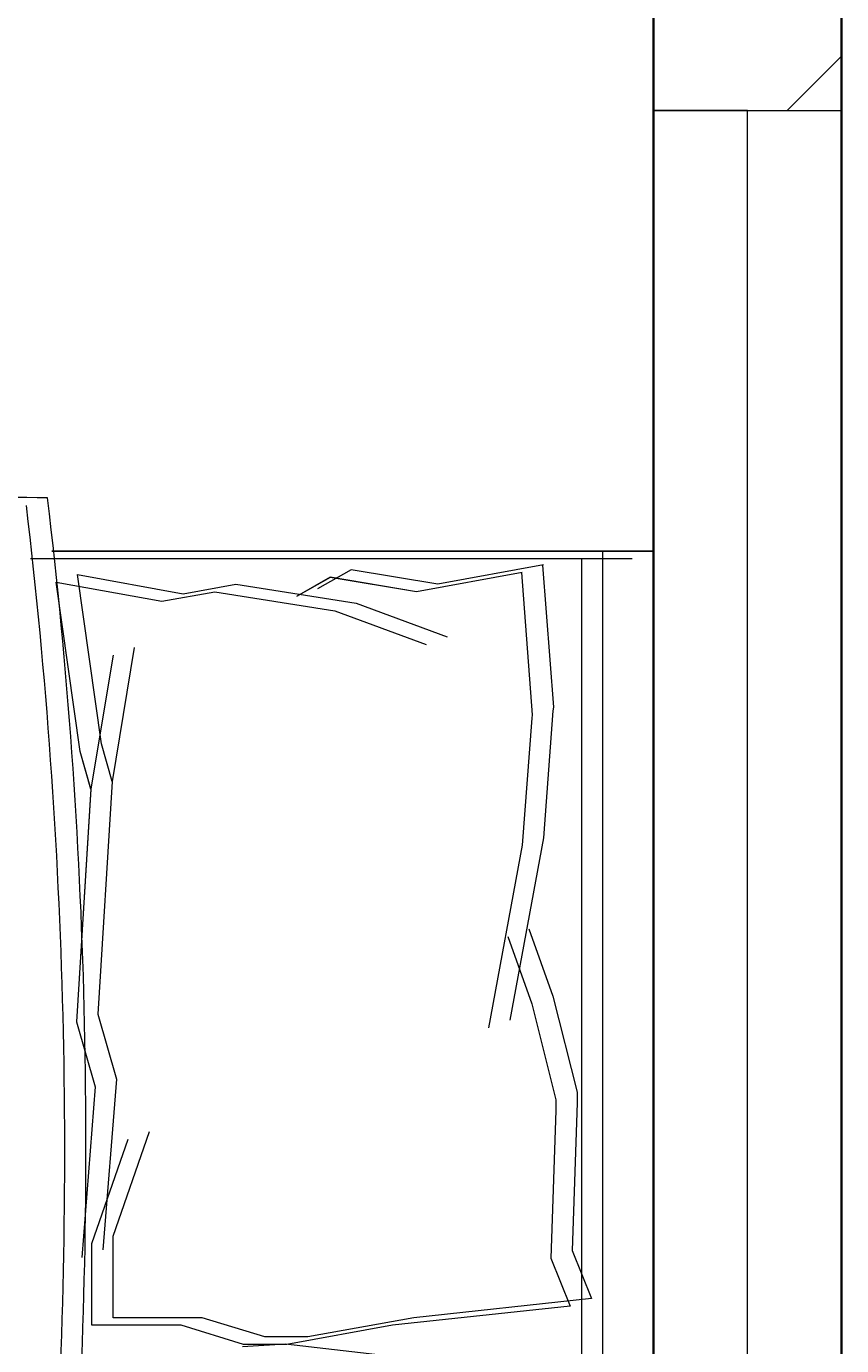
# Model space of a CAD drawing. Units: inches. Extents: x 1962 to 2771, y 1245 to 2660.
# Tile 77 of 114: x 2641 to 2661, y 2051 to 2082. Entities that reach past the tile are written whole.
import ezdxf

# ---------------------------------------------------------------- set-up
doc = ezdxf.new("R2010")
doc.units = ezdxf.units.IN
for name, color, linetype, lineweight in [('A-ANNO-DIMS', 2, 'Continuous', 18), ('A-FURN', 8, 'Continuous', 13), ('A-GLAZ', 4, 'Continuous', 18), ('A-WALL', 7, 'Continuous', 35), ('A-WALL-PATT', 252, 'Continuous', 13)]:
    doc.layers.add(name, color=color, linetype=linetype, lineweight=lineweight)
doc.styles.get("Standard").update_dxf_attribs({"font": 'arial.ttf'})
doc.dimstyles.get("Standard").update_dxf_attribs({"dimtxt": 0.18, "dimasz": 0.18, "dimexe": 0.18, "dimexo": 0.0625, "dimgap": 0.09, "dimtad": 0, "dimtih": 1, "dimtoh": 1, "dimdec": 4, "dimzin": 0, "dimdsep": 46, "dimtxsty": 'Standard', "dimcen": 0.09, "dimadec": 0, "dimazin": 0, "dimtfac": 1, "dimtdec": 4, "dimtofl": 0, "dimtmove": 0, "dimatfit": 3, "dimfxl": 1, "dimtolj": 1, "dimtzin": 0, "dimarcsym": 0})

# ---------------------------------------------------------------- blocks, each defined once
blk = doc.blocks.new('BED-PLAN')
for p, q in [((0, 2.764), (0, 40.751)), ((1.219, 2.764), (1.219, 40.752)), ((1.219, 2.763), (1.219, 40.751)), ((1.727, 2.945), (1.727, 40.933)), ((1.727, 2.945), (1.727, 40.933)), ((6.254, 22.046), (8.806, 21.745)), ((6.254, 22.046), (8.806, 21.745)), ((8.806, 21.745), (9.838, 21.81)), ((8.806, 21.745), (9.838, 21.81)), ((5.739, 21.114), (8.268, 21.574)), ((5.739, 21.114), (8.268, 21.574)), ((6.247, 21.296), (8.776, 21.755)), ((6.247, 21.296), (8.776, 21.755)), ((8.268, 21.574), (9.302, 21.574)), ((8.268, 21.574), (9.302, 21.574)), ((8.776, 21.755), (9.81, 21.755)), ((8.776, 21.755), (9.81, 21.755)), ((9.302, 21.574), (10.796, 21.114)), ((9.302, 21.574), (10.796, 21.114)), ((9.81, 21.755), (11.304, 21.296)), ((9.81, 21.755), (11.304, 21.296)), ((1.995, 20.836), (6.247, 21.296)), ((1.995, 20.836), (6.247, 21.296)), ((11.304, 21.296), (13.436, 21.296)), ((11.304, 21.296), (13.436, 21.296)), ((13.436, 21.296), (13.436, 19.342)), ((13.436, 21.296), (13.436, 19.342)), ((1.487, 20.655), (5.739, 21.114)), ((1.487, 20.654), (5.739, 21.114)), ((10.796, 21.114), (12.927, 21.114)), ((10.796, 21.114), (12.927, 21.114)), ((12.927, 21.114), (12.927, 19.161)), ((12.927, 21.114), (12.927, 19.161)), ((1.946, 19.506), (1.487, 20.655)), ((1.946, 19.505), (1.487, 20.654)), ((2.455, 19.687), (1.995, 20.836)), ((2.455, 19.687), (1.995, 20.836)), ((2.34, 16.153), (2.455, 19.687)), ((2.34, 16.153), (2.455, 19.687)), ((13.361, 15.591), (13.682, 19.67)), ((13.361, 15.591), (13.682, 19.67)), ((1.831, 15.972), (1.946, 19.506)), ((1.831, 15.972), (1.946, 19.505)), ((13.436, 19.342), (12.568, 16.843)), ((13.436, 19.342), (12.568, 16.843)), ((12.853, 15.409), (13.173, 19.489)), ((12.853, 15.409), (13.173, 19.488)), ((12.927, 19.161), (12.06, 16.661)), ((12.927, 19.161), (12.06, 16.661)), ((2.34, 15.898), (2.34, 16.153)), ((2.34, 15.897), (2.34, 16.153)), ((1.831, 15.716), (1.831, 15.972)), ((1.831, 15.716), (1.831, 15.972)), ((2.914, 13.6), (2.34, 15.898)), ((2.914, 13.599), (2.34, 15.897)), ((2.406, 13.418), (1.831, 15.716)), ((2.406, 13.418), (1.831, 15.716)), ((13.804, 14.033), (13.361, 15.591)), ((13.804, 14.032), (13.361, 15.591)), ((13.296, 13.851), (12.853, 15.409)), ((13.296, 13.851), (12.853, 15.409)), ((2.636, 9.626), (3.44, 13.993)), ((2.636, 9.626), (3.44, 13.992)), ((3.144, 9.808), (3.949, 14.174)), ((3.144, 9.807), (3.949, 14.174)), ((13.461, 8.461), (13.804, 14.033)), ((13.461, 8.46), (13.804, 14.032)), ((3.489, 11.991), (2.914, 13.6)), ((3.489, 11.991), (2.914, 13.599)), ((12.953, 8.279), (13.296, 13.851)), ((12.953, 8.279), (13.296, 13.851)), ((2.981, 11.809), (2.406, 13.418)), ((2.981, 11.809), (2.406, 13.418)), ((2.914, 6.768), (3.144, 9.808)), ((2.914, 6.768), (3.144, 9.807)), ((2.406, 6.587), (2.636, 9.626)), ((2.406, 6.587), (2.636, 9.626)), ((12.423, 5.074), (12.953, 8.279)), ((12.423, 5.074), (12.953, 8.279)), ((12.931, 5.256), (13.461, 8.461)), ((12.931, 5.255), (13.461, 8.46)), ((12.953, 8.279), (13.21, 7.378)), ((12.953, 8.279), (13.21, 7.378)), ((13.461, 8.461), (13.718, 7.56)), ((13.461, 8.46), (13.718, 7.56)), ((13.21, 7.378), (13.784, 3.327)), ((13.21, 7.378), (13.784, 3.327)), ((13.718, 7.56), (14.292, 3.509)), ((13.718, 7.56), (14.292, 3.508)), ((2.9, 6.685), (2.914, 6.768)), ((2.9, 6.684), (2.914, 6.768)), ((3.162, 3.282), (2.9, 6.685)), ((3.162, 3.282), (2.9, 6.684)), ((2.392, 6.503), (2.406, 6.587)), ((2.392, 6.503), (2.406, 6.587)), ((2.653, 3.1), (2.392, 6.503)), ((2.653, 3.1), (2.392, 6.503)), ((7.118, 4.016), (4.935, 4.821)), ((7.118, 4.016), (4.935, 4.821)), ((7.626, 4.198), (5.443, 5.002)), ((7.626, 4.198), (5.443, 5.002)), ((10.5, 3.738), (7.626, 4.198)), ((10.5, 3.738), (7.626, 4.198)), ((9.991, 3.557), (7.118, 4.016)), ((9.992, 3.557), (7.118, 4.016)), ((7.741, 3.394), (8.546, 3.853)), ((7.741, 3.393), (8.546, 3.853)), ((11.764, 3.968), (10.5, 3.738)), ((11.764, 3.968), (10.5, 3.738)), ((14.292, 3.509), (11.764, 3.968)), ((14.292, 3.508), (11.764, 3.968)), ((2.636, 3.097), (5.164, 3.557)), ((2.636, 3.097), (5.164, 3.557)), ((3.144, 3.279), (5.673, 3.738)), ((3.144, 3.279), (5.673, 3.738)), ((5.164, 3.557), (7.233, 3.212)), ((5.164, 3.557), (7.233, 3.212)), ((5.673, 3.738), (7.741, 3.394)), ((5.673, 3.738), (7.741, 3.393)), ((7.233, 3.212), (8.038, 3.672)), ((7.233, 3.212), (8.038, 3.672)), ((11.256, 3.787), (9.991, 3.557)), ((11.256, 3.786), (9.992, 3.557)), ((13.784, 3.327), (11.256, 3.787)), ((13.784, 3.327), (11.256, 3.786)), ((14.904, 2.945), (0.508, 2.945)), ((14.904, 2.945), (0.508, 2.945)), ((14.396, 2.764), (0, 2.764)), ((14.396, 2.763), (0, 2.763))]:
    blk.add_line(p, q)
for centre, radius, start, end in [((144.711, 16.979), 131.131, 176.08655, 186.78213), ((144.711, 16.979), 131.131, 176.08655, 186.78213), ((145.219, 17.161), 131.131, 176.08655, 186.78213), ((145.219, 17.161), 131.131, 176.08655, 186.78213), ((15.974, 67.695), 66.218, 268.72178, 275.60397), ((15.974, 67.695), 66.218, 268.72178, 275.60397)]:
    blk.add_arc(centre, radius, start, end)
blk = doc.blocks.new('WIN-60IN-A')
for p, q in [((2.25, 60), (2.25, 0)), ((2.25, 0), (0, 0)), ((0, 0), (4.5, 0))]:
    blk.add_line(p, q)
blk = doc.blocks.new('*D40')
at = {"layer": 'A-ANNO-DIMS', "color": 0, "lineweight": -2, "transparency": 16777216}
for p, q in [((2072.02, 2033.906), (2072.02, 2583.474)), ((2072.2, 2583.294), (2366.02, 2583.294)), ((2660.627, 2583.294), (2366.808, 2583.294)), ((2660.807, 2524.406), (2660.807, 2583.474))]:
    blk.add_line(p, q, dxfattribs=at)
at = {"layer": 'A-ANNO-DIMS', "color": 0, "transparency": 16777216}
for points in [[(2072.2, 2583.324), (2072.2, 2583.264), (2072.02, 2583.294)], [(2660.627, 2583.324), (2660.627, 2583.264), (2660.807, 2583.294)]]:
    blk.add_solid(points, dxfattribs=at)
at = {"layer": 'Defpoints', "color": 0, "transparency": 16777216}
for p in [(2660.807, 2583.294), (2660.807, 2524.344), (2072.02, 2033.844)]:
    blk.add_point(p, dxfattribs=at)
at = {"layer": 'A-ANNO-DIMS', "color": 0, "transparency": 16777216, "insert": (2366.414, 2583.294), "char_height": 0.18, "attachment_point": 5}
blk.add_mtext('\\A1;588.8', dxfattribs=at)

msp = doc.modelspace()

# ---------------------------------------------------------------- hatches: boundary and pattern name
at = {"layer": 'A-WALL-PATT'}
h = msp.add_hatch(dxfattribs=at)
h.set_pattern_fill('ANSI32', color=256)
h.paths.add_polyline_path([(2090.8074, 2467.3437), (2141.6481, 2467.3437), (2141.6481, 2469.5937), (2141.6481, 2471.8437), (2086.3074, 2471.8437), (2086.3074, 2422.5333), (2090.8074, 2422.5333)])
h.paths.add_polyline_path([(2282.7664, 2471.8437), (2204.8982, 2471.8437), (2204.8982, 2467.3437), (2234.8074, 2467.3437), (2234.8074, 2311.3437), (2228.7492, 2311.3437), (2228.7492, 2306.8437), (2234.8074, 2306.8437), (2331.9227, 2306.8437), (2331.9227, 2309.0937), (2331.9227, 2311.3437), (2239.3074, 2311.3437), (2239.3074, 2467.3437), (2282.7664, 2467.3437), (2282.7664, 2469.5937)])
h.paths.add_polyline_path([(2471.4531, 2519.8437), (2552.011, 2519.8437), (2564.3996, 2519.8437), (2564.3996, 2511.1389), (2568.8996, 2511.1389), (2568.8996, 2524.3437), (2466.9531, 2524.3437), (2466.9531, 2471.8437), (2450.0749, 2471.8437), (2446.4672, 2471.8437), (2446.4672, 2467.3437), (2450.0749, 2467.3437), (2475.9988, 2467.3437), (2475.9988, 2469.5937), (2475.9988, 2471.8437), (2471.4531, 2471.8437)])
h.paths.add_polyline_path([(2575.2231, 2469.5937), (2575.2231, 2471.8437), (2568.8996, 2471.8437), (2568.8996, 2487.1389), (2564.3996, 2487.1389), (2564.3996, 2471.8437), (2556.511, 2471.8437), (2499.2904, 2471.8437), (2499.2904, 2467.3437), (2507.8074, 2467.3437), (2507.8074, 2311.3437), (2414.863, 2311.3437), (2414.863, 2306.8437), (2512.3074, 2306.8437), (2517.0114, 2306.8437), (2517.0114, 2309.0937), (2517.0114, 2311.3437), (2512.3074, 2311.3437), (2512.3074, 2467.3437), (2575.2231, 2467.3437)])
h.paths.add_polyline_path([(2660.8074, 2471.8437), (2600.9602, 2471.8437), (2600.9602, 2467.3437), (2656.3074, 2467.3437), (2656.3074, 2432.5704), (2660.8074, 2432.5704)])
h.paths.add_polyline_path([(2660.8074, 2372.5704), (2656.3074, 2372.5704), (2656.3074, 2311.3437), (2600.276, 2311.3437), (2600.276, 2309.0937), (2600.276, 2306.8437), (2656.3074, 2306.8437), (2656.3074, 2296.2593), (2660.8074, 2296.2593)])
h.paths.add_polyline_path([(2572.3074, 2306.8437), (2577.1385, 2306.8437), (2577.1385, 2311.3437), (2551.082, 2311.3437), (2551.082, 2306.8437), (2567.8074, 2306.8437), (2567.8074, 2258.8437), (2540.0574, 2258.8437), (2540.0574, 2256.5937), (2540.0574, 2254.3437), (2567.8074, 2254.3437), (2656.3074, 2254.3437), (2656.3074, 2236.9085), (2660.8074, 2236.9085), (2660.8074, 2272.2593), (2656.3074, 2272.2593), (2656.3074, 2258.8437), (2572.3074, 2258.8437)])
h.paths.add_polyline_path([(2512.3074, 2254.3437), (2518.8716, 2254.3437), (2518.8716, 2256.5937), (2518.8716, 2258.8437), (2507.8074, 2258.8437), (2507.8074, 2177.8437), (2567.8074, 2177.8437), (2567.8074, 2172.9628), (2572.3074, 2172.9628), (2572.3074, 2177.8437), (2656.3074, 2177.8437), (2656.3074, 2166.4846), (2660.8074, 2166.4846), (2660.8074, 2200.9085), (2656.3074, 2200.9085), (2656.3074, 2182.3437), (2512.3074, 2182.3437)])
h.paths.add_polyline_path([(2656.3074, 2129.8437), (2572.3074, 2129.8437), (2572.3074, 2150.3044), (2570.0574, 2150.3044), (2567.8074, 2150.3044), (2567.8074, 2129.8437), (2507.8074, 2129.8437), (2507.8074, 2116.3027), (2510.0574, 2116.3027), (2512.3074, 2116.3027), (2512.3074, 2125.3437), (2567.8074, 2125.3437), (2572.3074, 2125.3437), (2656.3074, 2125.3437)])
h.paths.add_polyline_path([(2090.8074, 2362.5333), (2086.3074, 2362.5333), (2086.3074, 2298.6242), (2090.8074, 2298.6242), (2090.8074, 2306.8437), (2174.8074, 2306.8437), (2174.8074, 2286.4178), (2179.3074, 2286.4178), (2179.3074, 2306.8437), (2192.8641, 2306.8437), (2192.8641, 2309.0937), (2192.8641, 2311.3437), (2090.8074, 2311.3437)])
h.paths.add_polyline_path([(2209.156, 2258.8437), (2179.3074, 2258.8437), (2179.3074, 2263.2236), (2177.0574, 2263.2236), (2174.8074, 2263.2236), (2174.8074, 2258.8437), (2090.8074, 2258.8437), (2090.8074, 2274.6242), (2086.3074, 2274.6242), (2086.3074, 2238.2967), (2088.5574, 2238.2967), (2090.8074, 2238.2967), (2090.8074, 2254.3437), (2209.156, 2254.3437)])
h.paths.add_polyline_path([(2090.8074, 2177.8437), (2234.8074, 2177.8437), (2234.8074, 2173.1428), (2239.3074, 2173.1428), (2239.3074, 2258.8437), (2230.8442, 2258.8437), (2230.8442, 2256.5937), (2230.8442, 2254.3437), (2234.8074, 2254.3437), (2234.8074, 2182.3437), (2090.8074, 2182.3437), (2090.8074, 2202.2967), (2086.3074, 2202.2967), (2086.3074, 2140.0389), (2090.8074, 2140.0389)])
h.paths.add_polyline_path([(2090.8074, 2080.0389), (2086.3074, 2080.0389), (2086.3074, 2033.8437), (2090.8074, 2033.8437)], flags=17)
h.paths.add_polyline_path([(2244.9405, 2033.8437), (2239.3074, 2033.8437), (2239.3074, 2142.0665), (2237.2592, 2142.0665), (2234.8074, 2142.0665), (2234.8074, 2033.8437), (2090.8074, 2033.8437), (2076.5204, 2033.8437), (2072.0204, 2033.8437), (2072.0204, 2000.4493), (2076.5204, 2000.4493), (2076.5204, 2029.3437), (2090.8074, 2029.3437), (2244.9405, 2029.3437), (2244.9405, 2031.5937)])
h.paths.add_polyline_path([(2234.8074, 1933.3437), (2076.5204, 1933.3437), (2076.5204, 1952.4493), (2074.2704, 1952.4493), (2072.0204, 1952.4493), (2072.0204, 1933.3437), (2072.0204, 1928.8437), (2234.8074, 1928.8437)])
h.paths.add_polyline_path([(2090.8074, 1928.8437), (2086.3074, 1928.8437), (2086.3074, 1906.5013), (2090.8074, 1906.5013)])
h.paths.add_polyline_path([(2090.8074, 1846.5013), (2086.3074, 1846.5013), (2086.3074, 1769.9917), (2088.5574, 1769.9917), (2090.8074, 1769.9917), (2090.8074, 1780.3437), (2234.8074, 1780.3437), (2234.8074, 1708.3437), (2230.3764, 1708.3437), (2230.3764, 1703.8437), (2239.3074, 1703.8437), (2239.3074, 1792.6669), (2237.0574, 1792.6669), (2234.8074, 1792.6669), (2234.8074, 1784.8437), (2090.8074, 1784.8437)])
h.paths.add_polyline_path([(2239.3074, 1928.8437), (2244.9405, 1928.8437), (2244.9405, 1931.0937), (2244.9405, 1933.3437), (2234.8074, 1933.3437), (2234.8074, 1928.8437), (2234.8074, 1825.5949), (2239.3074, 1825.5949)])
h.paths.add_polyline_path([(2148.0425, 1649.0937), (2148.0425, 1651.3437), (2090.8074, 1651.3437), (2090.8074, 1646.8437), (2148.0425, 1646.8437)], flags=0)
h.paths.add_polyline_path([(2207.5601, 1708.3437), (2090.8074, 1708.3437), (2090.8074, 1703.8437), (2174.8074, 1703.8437), (2174.8074, 1651.3437), (2170.4457, 1651.3437), (2170.4457, 1646.8437), (2195.9924, 1646.8437), (2195.9924, 1649.0937), (2195.9924, 1651.3437), (2179.3074, 1651.3437), (2179.3074, 1703.8437), (2207.5601, 1703.8437), (2207.5601, 1706.0937)])
h.paths.add_polyline_path([(2090.8074, 1733.9917), (2086.3074, 1733.9917), (2086.3074, 1696.1032), (2088.5574, 1696.1032), (2090.8074, 1696.1032)])
h.paths.add_polyline_path([(2090.8074, 1672.1032), (2086.3074, 1672.1032), (2086.3074, 1600.3335), (2090.8074, 1600.3335)])
h.paths.add_polyline_path([(2090.8074, 1540.3335), (2086.3074, 1540.3335), (2086.3074, 1486.3437), (2139.6766, 1486.3437), (2139.6766, 1490.8437), (2090.8074, 1490.8437)])
h.paths.add_polyline_path([(2302.3876, 1490.8437), (2239.3074, 1490.8437), (2239.3074, 1646.8437), (2335.9994, 1646.8437), (2335.9994, 1651.3437), (2229.884, 1651.3437), (2229.884, 1646.8437), (2234.8074, 1646.8437), (2234.8074, 1490.8437), (2202.7103, 1490.8437), (2202.7103, 1488.5937), (2202.7103, 1486.3437), (2275.0699, 1486.3437), (2275.0699, 1475.772), (2279.5699, 1475.772), (2279.5699, 1486.3437), (2302.3876, 1486.3437)])
h.paths.add_polyline_path([(2279.5699, 1451.772), (2275.0699, 1451.772), (2275.0699, 1438.3437), (2174.8074, 1438.3437), (2174.8074, 1486.3437), (2179.7922, 1486.3437), (2179.7922, 1490.8437), (2163.3585, 1490.8437), (2163.3585, 1488.5937), (2163.3585, 1486.3437), (2170.3074, 1486.3437), (2170.3074, 1433.8437), (2279.5699, 1433.8437)])
h.paths.add_polyline_path([(2427.2363, 1490.8437), (2375.8074, 1490.8437), (2375.8074, 1646.8437), (2381.6401, 1646.8437), (2381.6401, 1651.3437), (2365.887, 1651.3437), (2365.887, 1649.0937), (2365.887, 1646.8437), (2371.3074, 1646.8437), (2371.3074, 1490.8437), (2327.5627, 1490.8437), (2327.5627, 1488.5937), (2327.5627, 1486.3437), (2371.3074, 1486.3437), (2371.3074, 1433.8437), (2375.8074, 1433.8437), (2375.8074, 1486.3437), (2427.2363, 1486.3437)])
h.paths.add_polyline_path([(2512.3074, 1646.8437), (2519.4351, 1646.8437), (2519.4351, 1649.0937), (2519.4351, 1651.3437), (2507.8074, 1651.3437), (2416.0063, 1651.3437), (2416.0063, 1649.0937), (2416.0063, 1646.8437), (2507.8074, 1646.8437), (2507.8074, 1490.8437), (2497.0532, 1490.8437), (2497.0532, 1488.5937), (2497.0532, 1486.3437), (2574.9344, 1486.3437), (2574.9344, 1476.0181), (2579.4344, 1476.0181), (2579.4344, 1486.3437), (2584.4872, 1486.3437), (2584.3074, 1490.8437), (2512.3074, 1490.8437)])
h.paths.add_polyline_path([(2470.5091, 1486.3437), (2473.9767, 1486.3437), (2473.9767, 1490.8437), (2449.6605, 1490.8437), (2449.6605, 1488.5937), (2449.6605, 1486.3437), (2466.0091, 1486.3437), (2466.0091, 1433.8437), (2470.5091, 1433.8437), (2579.4344, 1433.8437), (2579.4344, 1452.0181), (2574.9344, 1452.0181), (2574.9344, 1438.3437), (2554.5091, 1438.3437), (2470.5091, 1438.3437)])
h.paths.add_polyline_path([(2656.3074, 1490.8437), (2611.86, 1490.8437), (2611.86, 1486.3437), (2656.3074, 1486.3437)])
h.paths.add_polyline_path([(2660.8074, 1532.7007), (2658.5574, 1532.7007), (2656.3074, 1532.7007), (2656.3074, 1486.3437), (2660.8074, 1486.3437)])
h.paths.add_polyline_path([(2660.8074, 1664.9663), (2656.3074, 1664.9663), (2656.3074, 1651.3437), (2602.2313, 1651.3437), (2602.2313, 1646.8437), (2656.3074, 1646.8437), (2656.3074, 1592.7007), (2660.8074, 1592.7007)])
h.paths.add_polyline_path([(2660.8074, 1724.5221), (2656.3074, 1724.5221), (2656.3074, 1703.8437), (2542.4725, 1703.8437), (2542.4725, 1699.3437), (2567.8074, 1699.3437), (2567.8074, 1651.3437), (2552.7766, 1651.3437), (2552.7766, 1649.0937), (2552.7766, 1646.8437), (2577.2878, 1646.8437), (2577.2878, 1649.0937), (2577.2878, 1651.3437), (2572.3074, 1651.3437), (2572.3074, 1699.3437), (2656.3074, 1699.3437), (2656.3074, 1688.9663), (2660.8074, 1688.9663)])
h.paths.add_polyline_path([(2660.8074, 1880.6524), (2656.3074, 1880.6524), (2656.3074, 1832.8437), (2512.3074, 1832.8437), (2512.3074, 1837.8959), (2507.8074, 1837.8959), (2507.8074, 1828.3437), (2567.8074, 1828.3437), (2567.8074, 1804.3437), (2572.3074, 1804.3437), (2572.3074, 1828.3437), (2656.3074, 1828.3437), (2656.3074, 1818.6778), (2660.8074, 1818.6778)])
h.paths.add_polyline_path([(2660.8074, 1794.6778), (2656.3074, 1794.6778), (2656.3074, 1780.3437), (2572.3074, 1780.3437), (2572.3074, 1783.0303), (2570.0574, 1783.0303), (2567.8074, 1783.0303), (2567.8074, 1780.3437), (2507.8074, 1780.3437), (2507.8074, 1699.3437), (2517.8858, 1699.3437), (2517.8858, 1701.5937), (2517.8858, 1703.8437), (2512.3074, 1703.8437), (2512.3074, 1775.8437), (2656.3074, 1775.8437), (2656.3074, 1760.5221), (2660.8074, 1760.5221)])
h.paths.add_polyline_path([(2660.8074, 1981.3437), (2660.8074, 2020.2808), (2658.5574, 2020.2808), (2656.3074, 2020.2808), (2656.3074, 1981.3437), (2512.3074, 1981.3437), (2512.3074, 2086.6996), (2507.8074, 2086.6996), (2507.8074, 1981.3437), (2375.8074, 1981.3437), (2375.8074, 1986.8505), (2373.5574, 1986.8505), (2371.3074, 1986.8505), (2371.3074, 1973.2607), (2375.8074, 1973.2607), (2375.8074, 1976.8437), (2507.8074, 1976.8437), (2507.8074, 1865.4281), (2510.0574, 1865.4281), (2512.3074, 1865.4281), (2512.3074, 1976.8437), (2660.8074, 1976.8437)])
h.paths.add_polyline_path([(2375.8074, 1940.297), (2373.5574, 1940.297), (2371.3074, 1940.297), (2371.3074, 1933.3437), (2278.4434, 1933.3437), (2278.4434, 1928.8437), (2371.3074, 1928.8437), (2371.3074, 1651.3437), (2375.8074, 1651.3437)])
h.paths.add_polyline_path([(2660.8074, 1976.8437), (2656.3074, 1976.8437), (2656.3074, 1940.6524), (2660.8074, 1940.6524)], flags=17)
h.paths.add_polyline_path([(2660.8074, 2142.4846), (2656.3074, 2142.4846), (2656.3074, 2080.2808), (2660.8074, 2080.2808)])
h.paths.add_polyline_path([(2381.4189, 2311.3437), (2375.8074, 2311.3437), (2375.8074, 2467.3437), (2424.7242, 2467.3437), (2424.7242, 2469.5937), (2424.7242, 2471.8437), (2375.8074, 2471.8437), (2375.8074, 2524.3437), (2371.3074, 2524.3437), (2371.3074, 2471.8437), (2307.2097, 2471.8437), (2307.2097, 2467.3437), (2371.3074, 2467.3437), (2371.3074, 2311.3437), (2366.8901, 2311.3437), (2366.8901, 2306.8437), (2371.3074, 2306.8437), (2371.3074, 2033.8437), (2279.6589, 2033.8437), (2279.6589, 2029.3437), (2371.3074, 2029.3437), (2371.3074, 2014.2598), (2375.8074, 2014.2598), (2375.8074, 2306.8437), (2381.4189, 2306.8437)])
h.paths.add_polyline_path([(2263.3074, 2524.3437), (2170.3074, 2524.3437), (2170.3074, 2519.8437), (2170.3074, 2471.8437), (2165.0312, 2471.8437), (2165.0312, 2467.3437), (2179.6721, 2467.3437), (2179.6721, 2469.5161), (2179.6721, 2471.8437), (2174.8074, 2471.8437), (2174.8074, 2519.8437), (2258.8074, 2519.8437), (2258.8074, 2511.6436), (2263.3074, 2511.6436)])
h.paths.add_polyline_path([(2245.0232, 1361.4123), (2492.9468, 1361.4123), (2492.9468, 1398.505), (2245.0232, 1398.505)], flags=9)
h.paths.add_polyline_path([(2388.1434, 2086.6936), (2425.0704, 2086.6936), (2425.0704, 2105.3509), (2388.1434, 2105.3509)], flags=9)
h.paths.add_polyline_path([(2404.922, 2242.6744), (2445.7337, 2242.6744), (2445.7337, 2261.3318), (2404.922, 2261.3318)], flags=9)
h.paths.add_polyline_path([(2269.4107, 2156.7935), (2306.3378, 2156.7935), (2306.3378, 2175.4508), (2269.4107, 2175.4508)], flags=9)
h.paths.add_polyline_path([(2269.3277, 2233.4343), (2306.2547, 2233.4343), (2306.2547, 2252.0917), (2269.3277, 2252.0917)], flags=9)
h.paths.add_polyline_path([(2431.6052, 2320.6922), (2470.4456, 2320.6922), (2470.4456, 2339.3495), (2431.6052, 2339.3495)], flags=25)
h.paths.add_polyline_path([(2249.6902, 2315.7608), (2288.5306, 2315.7608), (2288.5306, 2334.4182), (2249.6902, 2334.4182)], flags=25)
h.paths.add_polyline_path([(2096.9301, 2314.3181), (2135.7704, 2314.3181), (2135.7704, 2332.9755), (2096.9301, 2332.9755)], flags=25)
h.paths.add_polyline_path([(2134.3475, 2285.7089), (2161.4655, 2285.7089), (2161.4655, 2304.3662), (2134.3475, 2304.3662)], flags=9)
h.paths.add_polyline_path([(2126.5155, 2209.4076), (2159.9227, 2209.4076), (2159.9227, 2228.065), (2126.5155, 2228.065)], flags=25)
h.paths.add_polyline_path([(2110.5753, 2141.5299), (2149.4157, 2141.5299), (2149.4157, 2160.1872), (2110.5753, 2160.1872)], flags=25)
h.paths.add_polyline_path([(2249.8618, 1968.3317), (2286.3966, 1968.3317), (2286.3966, 1986.989), (2249.8618, 1986.989)], flags=9)
h.paths.add_polyline_path([(2395.9507, 1777.0051), (2436.7624, 1777.0051), (2436.7624, 1795.6625), (2395.9507, 1795.6625)], flags=9)
h.paths.add_polyline_path([(2398.5259, 1888.5651), (2435.0062, 1888.5651), (2435.0062, 1907.2224), (2398.5259, 1907.2224)], flags=25)
h.paths.add_polyline_path([(2259.3506, 1728.3559), (2296.2776, 1728.3559), (2296.2776, 1747.0132), (2259.3506, 1747.0132)], flags=9)
h.paths.add_polyline_path([(2271.3698, 1845.268), (2308.2968, 1845.268), (2308.2968, 1863.9253), (2271.3698, 1863.9253)], flags=9)
h.paths.add_polyline_path([(2120.9355, 1786.3027), (2159.7759, 1786.3027), (2159.7759, 1804.9601), (2120.9355, 1804.9601)], flags=25)
h.paths.add_polyline_path([(2121.3164, 1732.1043), (2154.7236, 1732.1043), (2154.7236, 1750.7616), (2121.3164, 1750.7616)], flags=25)
h.paths.add_polyline_path([(2118.3706, 1678.8997), (2147.5282, 1678.8997), (2147.5282, 1697.557), (2118.3706, 1697.557)], flags=25)
h.paths.add_polyline_path([(2385.9227, 1493.557), (2424.763, 1493.557), (2424.763, 1512.2143), (2385.9227, 1512.2143)], flags=25)
h.paths.add_polyline_path([(2248.7058, 1500.0256), (2287.5462, 1500.0256), (2287.5462, 1518.6829), (2248.7058, 1518.6829)], flags=25)
h.paths.add_polyline_path([(2104.1669, 1617.3771), (2143.0073, 1617.3771), (2143.0073, 1636.0344), (2104.1669, 1636.0344)], flags=9)
h.paths.add_polyline_path([(2096.0714, 1447.8824), (2137.3845, 1447.8824), (2137.3845, 1458.1859), (2096.0714, 1458.1859)], flags=9)
h.paths.add_polyline_path([(2180.6114, 1440.325), (2209.7689, 1440.325), (2209.7689, 1458.9823), (2180.6114, 1458.9823)], flags=25)
h.paths.add_polyline_path([(2316.1698, 1447.9637), (2357.4829, 1447.9637), (2357.4829, 1458.2673), (2316.1698, 1458.2673)], flags=9)
h.paths.add_polyline_path([(2397.6187, 1447.9637), (2438.9318, 1447.9637), (2438.9318, 1458.2673), (2397.6187, 1458.2673)], flags=9)
h.paths.add_polyline_path([(2473.0778, 1439.5953), (2502.2354, 1439.5953), (2502.2354, 1458.2527), (2473.0778, 1458.2527)], flags=25)
h.paths.add_polyline_path([(2589.7027, 1447.8819), (2631.0158, 1447.8819), (2631.0158, 1458.1855), (2589.7027, 1458.1855)], flags=9)
h.paths.add_polyline_path([(2522.4009, 1497.5285), (2561.2413, 1497.5285), (2561.2413, 1516.1859), (2522.4009, 1516.1859)], flags=25)
h.paths.add_polyline_path([(2579.6565, 1671.3482), (2608.8141, 1671.3482), (2608.8141, 1690.0056), (2579.6565, 1690.0056)], flags=25)
h.paths.add_polyline_path([(2544.7038, 1725.5064), (2578.1111, 1725.5064), (2578.1111, 1744.1637), (2544.7038, 1744.1637)], flags=25)
h.paths.add_polyline_path([(2578.1191, 1807.472), (2607.2766, 1807.472), (2607.2766, 1826.1293), (2578.1191, 1826.1293)], flags=25)
h.paths.add_polyline_path([(2595.0614, 1835.1839), (2633.9018, 1835.1839), (2633.9018, 1853.8413), (2595.0614, 1853.8413)], flags=25)
h.paths.add_polyline_path([(2567.0097, 2097.7035), (2605.8501, 2097.7035), (2605.8501, 2116.3609), (2567.0097, 2116.3609)], flags=9)
h.paths.add_polyline_path([(2586.644, 2134.6454), (2615.8015, 2134.6454), (2615.8015, 2153.3027), (2586.644, 2153.3027)], flags=9)
h.paths.add_polyline_path([(2544.6185, 2212.6783), (2578.0258, 2212.6783), (2578.0258, 2231.3356), (2544.6185, 2231.3356)], flags=25)
h.paths.add_polyline_path([(2577.0273, 2256.9023), (2606.1849, 2256.9023), (2606.1849, 2275.5597), (2577.0273, 2275.5597)], flags=24)
h.paths.add_polyline_path([(2605.2683, 2315.2821), (2644.1087, 2315.2821), (2644.1087, 2333.9395), (2605.2683, 2333.9395)], flags=25)
h.paths.add_polyline_path([(2583.1244, 2496.1815), (2624.4375, 2496.1815), (2624.4375, 2506.4851), (2583.1244, 2506.4851)], flags=9)
h.paths.add_polyline_path([(2474.761, 2497.0823), (2503.9185, 2497.0823), (2503.9185, 2515.7397), (2474.761, 2515.7397)], flags=25)
h.paths.add_polyline_path([(2387.5787, 2494.2563), (2428.902, 2494.2563), (2428.902, 2504.5598), (2387.5787, 2504.5598)], flags=9)
h.paths.add_polyline_path([(2300.1657, 2500.1564), (2341.4788, 2500.1564), (2341.4788, 2510.46), (2300.1657, 2510.46)], flags=25)
h.paths.add_polyline_path([(2176.8589, 2497.5843), (2206.0165, 2497.5843), (2206.0165, 2516.2416), (2176.8589, 2516.2416)], flags=25)
h.paths.add_polyline_path([(2097.4668, 2494.9762), (2138.7799, 2494.9762), (2138.7799, 2505.2798), (2097.4668, 2505.2798)], flags=9)

# ---------------------------------------------------------------- linework, layer by layer
at = {"layer": 'A-WALL'}
for p, q in [((2660.8074, 2471.8437), (2660.8074, 1976.8437)), ((2656.3074, 2177.8437), (2656.3074, 1981.3437))]:
    msp.add_line(p, q, dxfattribs=at)

# ---------------------------------------------------------------- block references
at = {"layer": 'A-FURN', "rotation": 180}
msp.add_blockref('BED-PLAN', (2656.3074, 2072.498), dxfattribs=at)
at = {"layer": 'A-GLAZ', "extrusion": (0, 0, -1), "zscale": -1, "rotation": 180}
msp.add_blockref('WIN-60IN-A', (-2656.3074, 2080.2808), dxfattribs=at)

# ---------------------------------------------------------------- dimensions: what is measured, and where the dimension line sits
at = {"layer": 'A-ANNO-DIMS'}
dim = msp.add_linear_dim(base=(2660.8074, 2583.2937), p1=(2072.0204, 2033.8437), p2=(2660.8074, 2524.3437), dimstyle='Standard', override={"dimdec": 1, "dimlfac": 1, "dimrnd": 0, "dimzin": 0, "dimdsep": 46, "dimlunit": 2}, dxfattribs=at)
dim.commit()
dim.dimension.update_dxf_attribs({"geometry": '*D40', "text_midpoint": (2366.4139, 2583.2937)})

doc.saveas('drawing.dxf')
